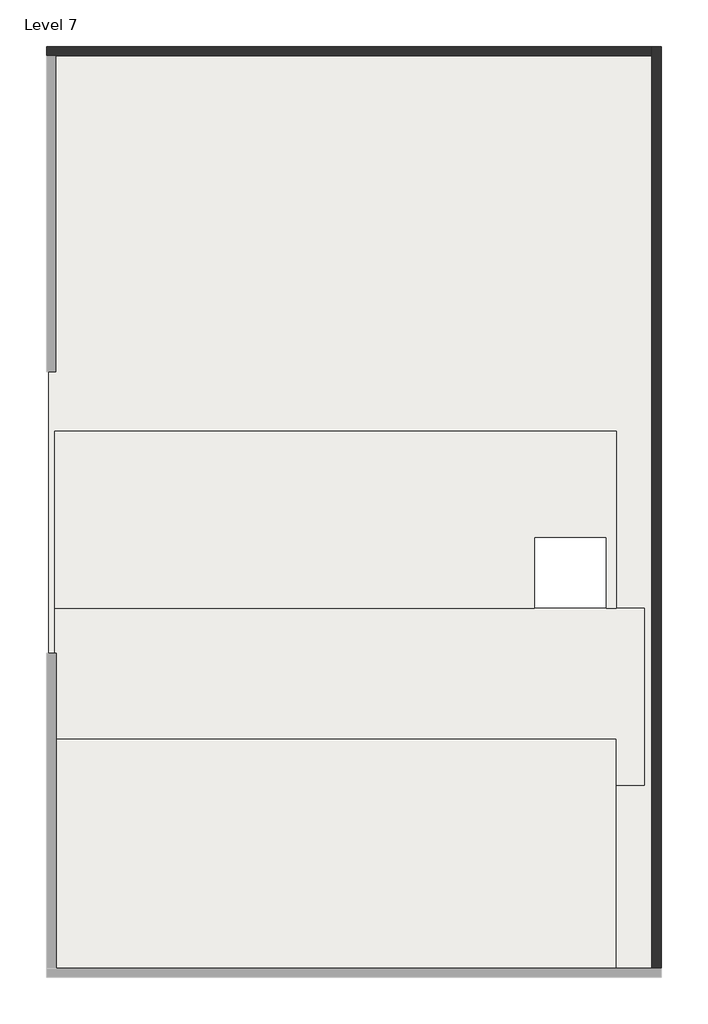
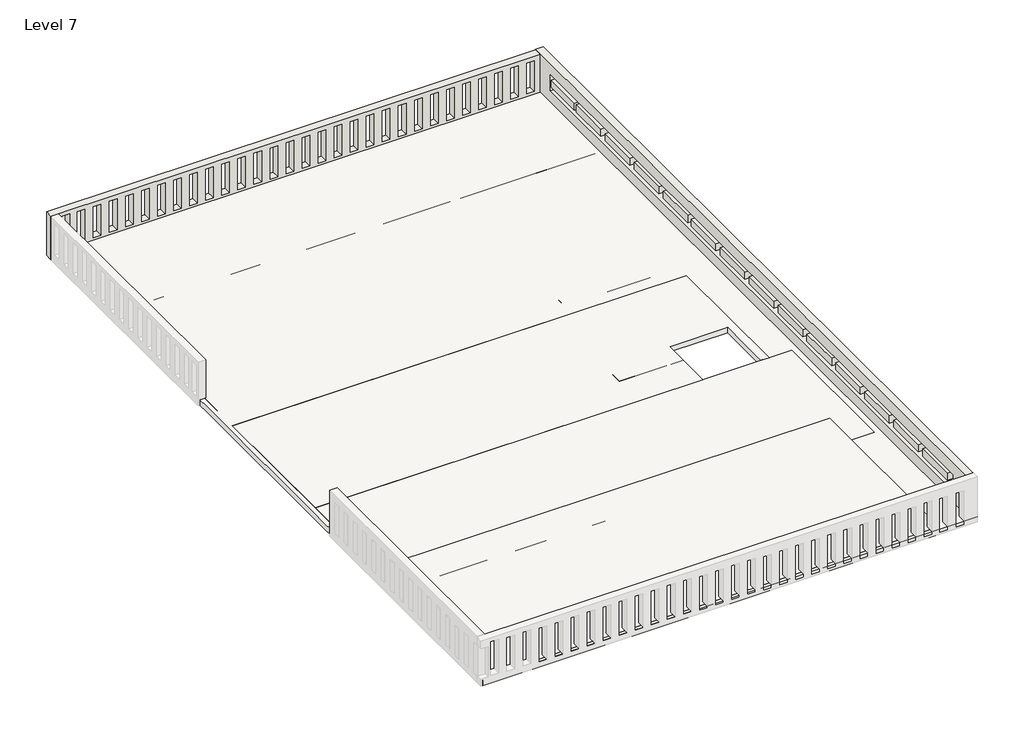
# One storey, part 2 of 2: 8 roofs, 2 walls.
"""IFC4 building model written with IfcOpenShell, lengths in millimetres."""

from ifc_helpers import new_model, si_unit, frame, origin, place, context, project, spatial, polyline, outline, extrude, faceted_brep, element, save

model = new_model("IFC4")

# Units and contexts
model_context = context("Model", 3, world=origin())
ifc_project = project(units=[si_unit("LENGTHUNIT", "METRE", prefix="MILLI")], contexts=[model_context])

# Site, building, storey
site = spatial("IfcSite", under=ifc_project)
building = spatial("IfcBuilding", under=site)
storey = spatial("IfcBuildingStorey", under=building, Name="Level 7", Elevation=18288.0)

# Roofs
placement = place(None, origin())
element("IfcRoof", 1, ObjectType="Generic - 12\"", at=placement, inside=storey, context=model_context, shape_type="SweptSolid", body=[
    extrude(outline(polyline([(-6354.2109037, 9427.2527313), (6498.1890963, 9427.2527313), (6498.1890963, 6506.6962251), (-6354.2109037, 6506.6962251), (-6354.2109037, 9427.2527313)])), frame((0.0, 0.0, 18288.0), z_axis=(0.0, 0.0, 1.0), x_axis=(1.0, 0.0, 0.0)), (0.0, 0.0, 1.0), 152.4),
])
element("IfcRoof", 2, ObjectType="Generic - 12\"", at=placement, inside=storey, context=model_context, shape_type="SweptSolid", body=[
    extrude(outline(polyline([(-6330.8013636, -2688.1037749), (6485.4890963, -2688.1037749), (6485.4890963, -6529.1251987), (-6330.8013636, -6529.1251987), (-6330.8013636, -2688.1037749)])), frame((0.0, 0.0, 18288.0), z_axis=(0.0, 0.0, 1.0), x_axis=(1.0, 0.0, 0.0)), (0.0, 0.0, 1.0), 152.4),
])
element("IfcRoof", 3, ObjectType="Generic - 12\"", at=placement, inside=storey, context=model_context, shape_type="SweptSolid", body=[
    extrude(outline(polyline([(-6354.2109037, -5532.9037749), (5863.1890963, -5532.9037749), (5863.1890963, -10612.9037749), (-6354.2109037, -10612.9037749), (-6354.2109037, -5532.9037749)])), frame((0.0, 0.0, 18288.0), z_axis=(0.0, 0.0, 1.0), x_axis=(1.0, 0.0, 0.0)), (0.0, 0.0, 1.0), 152.4),
])
element("IfcRoof", 4, ObjectType="Generic - 12\"", at=placement, inside=storey, context=model_context, shape_type="SweptSolid", body=[
    extrude(outline(polyline([(-6330.8013636, 6506.6962251), (5875.8890963, 6506.6962251), (5875.8890963, 1160.801054), (-6330.8013636, 1160.801054), (-6330.8013636, 6506.6962251)])), frame((0.0, 0.0, 18288.0), z_axis=(0.0, 0.0, 1.0), x_axis=(1.0, 0.0, 0.0)), (0.0, 0.0, 1.0), 152.4),
])
element("IfcRoof", 5, ObjectType="Generic - 12\"", at=placement, inside=storey, context=model_context, shape_type="SweptSolid", body=[
    extrude(outline(polyline([(-6330.8013636, 1160.801054), (5875.8890963, 1160.801054), (5875.8890963, -2688.1037749), (5659.9890963, -2688.1037749), (5659.9890963, -1138.7037749), (4097.8890963, -1138.7037749), (4097.8890963, -2688.1037749), (-6330.8013636, -2688.1037749), (-6330.8013636, 1160.801054)])), frame((0.0, 0.0, 18288.0), z_axis=(0.0, 0.0, 1.0), x_axis=(1.0, 0.0, 0.0)), (0.0, 0.0, 1.0), 152.4),
])
element("IfcRoof", 6, ObjectType="Generic - 12\"", at=placement, inside=storey, context=model_context, shape_type="SweptSolid", body=[
    extrude(outline(polyline([(2372.9046693, -1781.7441535), (2372.9046693, -1138.7037749), (4097.8890963, -1138.7037749), (4097.8890963, -1781.7441535), (2372.9046693, -1781.7441535)])), frame((0.0, 0.0, 18288.0), z_axis=(0.0, 0.0, 1.0), x_axis=(1.0, 0.0, 0.0)), (0.0, 0.0, 1.0), 152.4),
])
element("IfcRoof", 7, ObjectType="Generic - 12\"", at=placement, inside=storey, context=model_context, shape_type="SweptSolid", body=[
    extrude(outline(polyline([(5086.1735773, 1505.3140413), (2800.1735773, 1505.3140413), (2800.1735773, 1774.3862477), (5086.1735773, 1774.3862477), (5086.1735773, 1505.3140413)])), frame((0.0, 0.0, 18288.0), z_axis=(0.0, 0.0, 1.0), x_axis=(1.0, 0.0, 0.0)), (0.0, 0.0, 1.0), 152.4),
])
element("IfcRoof", 8, ObjectType="Generic - 12\"", at=placement, inside=storey, context=model_context, shape_type="SweptSolid", body=[
    extrude(outline(polyline([(6853.7890963, -10703.6694836), (-6455.8109037, -10703.6694836), (-6455.8109037, 9516.5962251), (6853.7890963, 9516.5962251), (6853.7890963, -10703.6694836)]), holes=[polyline([(5659.9890963, -1138.7037749), (4097.8890963, -1138.7037749), (4097.8890963, -2688.1037749), (5659.9890963, -2688.1037749), (5659.9890963, -1138.7037749)])]), frame((0.0, 0.0, 18288.0), z_axis=(0.0, 0.0, 1.0), x_axis=(1.0, 0.0, 0.0)), (0.0, 0.0, 1.0), 152.4),
])

# Walls
element("IfcWall", 9, ObjectType="Generic - 9\" w", at=placement, inside=storey, context=model_context, shape_type="Brep", body=[
    faceted_brep([(-6506.6109037, 9313.3962251, 18288.0), (-6303.4109037, 9313.3962251, 18288.0), (6650.5890963, 9313.3962251, 18288.0), (6650.5890963, 9313.3962251, 19521.0013439), (-6506.6109037, 9313.3962251, 19521.0013439), (-6506.6109037, 9313.3962251, 19520.2498043), (6294.9890963, 9313.3962251, 19391.3906419), (6498.1890963, 9313.3962251, 19391.3906419), (6498.1890963, 9313.3962251, 18512.6701562), (6294.9890963, 9313.3962251, 18512.6701562), (5863.1890963, 9313.3962251, 19391.3906419), (6066.3890963, 9313.3962251, 19391.3906419), (6066.3890963, 9313.3962251, 18512.6701562), (5863.1890963, 9313.3962251, 18512.6701562), (5431.3890963, 9313.3962251, 19391.3906419), (5634.5890963, 9313.3962251, 19391.3906419), (5634.5890963, 9313.3962251, 18512.6701562), (5431.3890963, 9313.3962251, 18512.6701562), (4999.5890963, 9313.3962251, 19391.3906419), (5202.7890963, 9313.3962251, 19391.3906419), (5202.7890963, 9313.3962251, 18512.6701562), (4999.5890963, 9313.3962251, 18512.6701562), (4567.7890963, 9313.3962251, 19391.3906419), (4770.9890963, 9313.3962251, 19391.3906419), (4770.9890963, 9313.3962251, 18512.6701562), (4567.7890963, 9313.3962251, 18512.6701562), (4135.9890963, 9313.3962251, 19391.3906419), (4339.1890963, 9313.3962251, 19391.3906419), (4339.1890963, 9313.3962251, 18512.6701562), (4135.9890963, 9313.3962251, 18512.6701562), (3704.1890963, 9313.3962251, 19391.3906419), (3907.3890963, 9313.3962251, 19391.3906419), (3907.3890963, 9313.3962251, 18512.6701562), (3704.1890963, 9313.3962251, 18512.6701562), (3272.3890963, 9313.3962251, 19391.3906419), (3475.5890963, 9313.3962251, 19391.3906419), (3475.5890963, 9313.3962251, 18512.6701562), (3272.3890963, 9313.3962251, 18512.6701562), (2840.5890963, 9313.3962251, 19391.3906419), (3043.7890963, 9313.3962251, 19391.3906419), (3043.7890963, 9313.3962251, 18512.6701562), (2840.5890963, 9313.3962251, 18512.6701562), (2408.7890963, 9313.3962251, 19391.3906419), (2611.9890963, 9313.3962251, 19391.3906419), (2611.9890963, 9313.3962251, 18512.6701562), (2408.7890963, 9313.3962251, 18512.6701562), (1976.9890963, 9313.3962251, 19391.3906419), (2180.1890963, 9313.3962251, 19391.3906419), (2180.1890963, 9313.3962251, 18512.6701562), (1976.9890963, 9313.3962251, 18512.6701562), (1545.1890963, 9313.3962251, 19391.3906419), (1748.3890963, 9313.3962251, 19391.3906419), (1748.3890963, 9313.3962251, 18512.6701562), (1545.1890963, 9313.3962251, 18512.6701562), (1113.3890963, 9313.3962251, 19391.3906419), (1316.5890963, 9313.3962251, 19391.3906419), (1316.5890963, 9313.3962251, 18512.6701562), (1113.3890963, 9313.3962251, 18512.6701562), (681.5890963, 9313.3962251, 19391.3906419), (884.7890963, 9313.3962251, 19391.3906419), (884.7890963, 9313.3962251, 18512.6701562), (681.5890963, 9313.3962251, 18512.6701562), (249.7890963, 9313.3962251, 19391.3906419), (452.9890963, 9313.3962251, 19391.3906419), (452.9890963, 9313.3962251, 18512.6701562), (249.7890963, 9313.3962251, 18512.6701562), (-182.0109037, 9313.3962251, 19391.3906419), (21.1890963, 9313.3962251, 19391.3906419), (21.1890963, 9313.3962251, 18512.6701562), (-182.0109037, 9313.3962251, 18512.6701562), (-613.8109037, 9313.3962251, 19391.3906419), (-410.6109037, 9313.3962251, 19391.3906419), (-410.6109037, 9313.3962251, 18512.6701562), (-613.8109037, 9313.3962251, 18512.6701562), (-1045.6109037, 9313.3962251, 19391.3906419), (-842.4109037, 9313.3962251, 19391.3906419), (-842.4109037, 9313.3962251, 18512.6701562), (-1045.6109037, 9313.3962251, 18512.6701562), (-1477.4109037, 9313.3962251, 19391.3906419), (-1274.2109037, 9313.3962251, 19391.3906419), (-1274.2109037, 9313.3962251, 18512.6701562), (-1477.4109037, 9313.3962251, 18512.6701562), (-1909.2109037, 9313.3962251, 19391.3906419), (-1706.0109037, 9313.3962251, 19391.3906419), (-1706.0109037, 9313.3962251, 18512.6701562), (-1909.2109037, 9313.3962251, 18512.6701562), (-2341.0109037, 9313.3962251, 19391.3906419), (-2137.8109037, 9313.3962251, 19391.3906419), (-2137.8109037, 9313.3962251, 18512.6701562), (-2341.0109037, 9313.3962251, 18512.6701562), (-2772.8109037, 9313.3962251, 19391.3906419), (-2569.6109037, 9313.3962251, 19391.3906419), (-2569.6109037, 9313.3962251, 18512.6701562), (-2772.8109037, 9313.3962251, 18512.6701562), (-3204.6109037, 9313.3962251, 19391.3906419), (-3001.4109037, 9313.3962251, 19391.3906419), (-3001.4109037, 9313.3962251, 18512.6701562), (-3204.6109037, 9313.3962251, 18512.6701562), (-3636.4109037, 9313.3962251, 19391.3906419), (-3433.2109037, 9313.3962251, 19391.3906419), (-3433.2109037, 9313.3962251, 18512.6701562), (-3636.4109037, 9313.3962251, 18512.6701562), (-4068.2109037, 9313.3962251, 19391.3906419), (-3865.0109037, 9313.3962251, 19391.3906419), (-3865.0109037, 9313.3962251, 18512.6701562), (-4068.2109037, 9313.3962251, 18512.6701562), (-4500.0109037, 9313.3962251, 19391.3906419), (-4296.8109037, 9313.3962251, 19391.3906419), (-4296.8109037, 9313.3962251, 18512.6701562), (-4500.0109037, 9313.3962251, 18512.6701562), (-4931.8109037, 9313.3962251, 19391.3906419), (-4728.6109037, 9313.3962251, 19391.3906419), (-4728.6109037, 9313.3962251, 18512.6701562), (-4931.8109037, 9313.3962251, 18512.6701562), (-5363.6109037, 9313.3962251, 19391.3906419), (-5160.4109037, 9313.3962251, 19391.3906419), (-5160.4109037, 9313.3962251, 18512.6701562), (-5363.6109037, 9313.3962251, 18512.6701562), (-5795.4109037, 9313.3962251, 19391.3906419), (-5592.2109037, 9313.3962251, 19391.3906419), (-5592.2109037, 9313.3962251, 18512.6701562), (-5795.4109037, 9313.3962251, 18512.6701562), (-6201.2539467, 9313.3962251, 19412.6599745), (-5998.0539467, 9313.3962251, 19412.6599745), (-5998.0539467, 9313.3962251, 18533.9394888), (-6201.2539467, 9313.3962251, 18533.9394888), (-6506.6109037, 9516.5962251, 18288.0), (-6506.6109037, 9516.5962251, 19521.0013439), (6650.5890963, 9516.5962251, 19521.0013439), (6650.5890963, 9516.5962251, 18288.0), (6294.9890963, 9516.5962251, 19391.3906419), (6294.9890963, 9516.5962251, 18512.6701562), (6498.1890963, 9516.5962251, 18512.6701562), (6498.1890963, 9516.5962251, 19391.3906419), (5863.1890963, 9516.5962251, 19391.3906419), (5863.1890963, 9516.5962251, 18512.6701562), (6066.3890963, 9516.5962251, 18512.6701562), (6066.3890963, 9516.5962251, 19391.3906419), (5431.3890963, 9516.5962251, 19391.3906419), (5431.3890963, 9516.5962251, 18512.6701562), (5634.5890963, 9516.5962251, 18512.6701562), (5634.5890963, 9516.5962251, 19391.3906419), (4999.5890963, 9516.5962251, 19391.3906419), (4999.5890963, 9516.5962251, 18512.6701562), (5202.7890963, 9516.5962251, 18512.6701562), (5202.7890963, 9516.5962251, 19391.3906419), (4567.7890963, 9516.5962251, 19391.3906419), (4567.7890963, 9516.5962251, 18512.6701562), (4770.9890963, 9516.5962251, 18512.6701562), (4770.9890963, 9516.5962251, 19391.3906419), (4135.9890963, 9516.5962251, 19391.3906419), (4135.9890963, 9516.5962251, 18512.6701562), (4339.1890963, 9516.5962251, 18512.6701562), (4339.1890963, 9516.5962251, 19391.3906419), (3704.1890963, 9516.5962251, 19391.3906419), (3704.1890963, 9516.5962251, 18512.6701562), (3907.3890963, 9516.5962251, 18512.6701562), (3907.3890963, 9516.5962251, 19391.3906419), (3272.3890963, 9516.5962251, 19391.3906419), (3272.3890963, 9516.5962251, 18512.6701562), (3475.5890963, 9516.5962251, 18512.6701562), (3475.5890963, 9516.5962251, 19391.3906419), (2840.5890963, 9516.5962251, 19391.3906419), (2840.5890963, 9516.5962251, 18512.6701562), (3043.7890963, 9516.5962251, 18512.6701562), (3043.7890963, 9516.5962251, 19391.3906419), (2408.7890963, 9516.5962251, 19391.3906419), (2408.7890963, 9516.5962251, 18512.6701562), (2611.9890963, 9516.5962251, 18512.6701562), (2611.9890963, 9516.5962251, 19391.3906419), (1976.9890963, 9516.5962251, 19391.3906419), (1976.9890963, 9516.5962251, 18512.6701562), (2180.1890963, 9516.5962251, 18512.6701562), (2180.1890963, 9516.5962251, 19391.3906419), (1545.1890963, 9516.5962251, 19391.3906419), (1545.1890963, 9516.5962251, 18512.6701562), (1748.3890963, 9516.5962251, 18512.6701562), (1748.3890963, 9516.5962251, 19391.3906419), (1113.3890963, 9516.5962251, 19391.3906419), (1113.3890963, 9516.5962251, 18512.6701562), (1316.5890963, 9516.5962251, 18512.6701562), (1316.5890963, 9516.5962251, 19391.3906419), (681.5890963, 9516.5962251, 19391.3906419), (681.5890963, 9516.5962251, 18512.6701562), (884.7890963, 9516.5962251, 18512.6701562), (884.7890963, 9516.5962251, 19391.3906419), (249.7890963, 9516.5962251, 19391.3906419), (249.7890963, 9516.5962251, 18512.6701562), (452.9890963, 9516.5962251, 18512.6701562), (452.9890963, 9516.5962251, 19391.3906419), (-182.0109037, 9516.5962251, 19391.3906419), (-182.0109037, 9516.5962251, 18512.6701562), (21.1890963, 9516.5962251, 18512.6701562), (21.1890963, 9516.5962251, 19391.3906419), (-613.8109037, 9516.5962251, 19391.3906419), (-613.8109037, 9516.5962251, 18512.6701562), (-410.6109037, 9516.5962251, 18512.6701562), (-410.6109037, 9516.5962251, 19391.3906419), (-1045.6109037, 9516.5962251, 19391.3906419), (-1045.6109037, 9516.5962251, 18512.6701562), (-842.4109037, 9516.5962251, 18512.6701562), (-842.4109037, 9516.5962251, 19391.3906419), (-1477.4109037, 9516.5962251, 19391.3906419), (-1477.4109037, 9516.5962251, 18512.6701562), (-1274.2109037, 9516.5962251, 18512.6701562), (-1274.2109037, 9516.5962251, 19391.3906419), (-1909.2109037, 9516.5962251, 19391.3906419), (-1909.2109037, 9516.5962251, 18512.6701562), (-1706.0109037, 9516.5962251, 18512.6701562), (-1706.0109037, 9516.5962251, 19391.3906419), (-2341.0109037, 9516.5962251, 19391.3906419), (-2341.0109037, 9516.5962251, 18512.6701562), (-2137.8109037, 9516.5962251, 18512.6701562), (-2137.8109037, 9516.5962251, 19391.3906419), (-2772.8109037, 9516.5962251, 19391.3906419), (-2772.8109037, 9516.5962251, 18512.6701562), (-2569.6109037, 9516.5962251, 18512.6701562), (-2569.6109037, 9516.5962251, 19391.3906419), (-3204.6109037, 9516.5962251, 19391.3906419), (-3204.6109037, 9516.5962251, 18512.6701562), (-3001.4109037, 9516.5962251, 18512.6701562), (-3001.4109037, 9516.5962251, 19391.3906419), (-3636.4109037, 9516.5962251, 19391.3906419), (-3636.4109037, 9516.5962251, 18512.6701562), (-3433.2109037, 9516.5962251, 18512.6701562), (-3433.2109037, 9516.5962251, 19391.3906419), (-4068.2109037, 9516.5962251, 19391.3906419), (-4068.2109037, 9516.5962251, 18512.6701562), (-3865.0109037, 9516.5962251, 18512.6701562), (-3865.0109037, 9516.5962251, 19391.3906419), (-4500.0109037, 9516.5962251, 19391.3906419), (-4500.0109037, 9516.5962251, 18512.6701562), (-4296.8109037, 9516.5962251, 18512.6701562), (-4296.8109037, 9516.5962251, 19391.3906419), (-4931.8109037, 9516.5962251, 19391.3906419), (-4931.8109037, 9516.5962251, 18512.6701562), (-4728.6109037, 9516.5962251, 18512.6701562), (-4728.6109037, 9516.5962251, 19391.3906419), (-5363.6109037, 9516.5962251, 19391.3906419), (-5363.6109037, 9516.5962251, 18512.6701562), (-5160.4109037, 9516.5962251, 18512.6701562), (-5160.4109037, 9516.5962251, 19391.3906419), (-5795.4109037, 9516.5962251, 19391.3906419), (-5795.4109037, 9516.5962251, 18512.6701562), (-5592.2109037, 9516.5962251, 18512.6701562), (-5592.2109037, 9516.5962251, 19391.3906419), (-6201.2539467, 9516.5962251, 19412.6599745), (-6201.2539467, 9516.5962251, 18533.9394888), (-5998.0539467, 9516.5962251, 18533.9394888), (-5998.0539467, 9516.5962251, 19412.6599745)], [[[0, 1, 2, 3, 4, 5], [6, 7, 8, 9], [10, 11, 12, 13], [14, 15, 16, 17], [18, 19, 20, 21], [22, 23, 24, 25], [26, 27, 28, 29], [30, 31, 32, 33], [34, 35, 36, 37], [38, 39, 40, 41], [42, 43, 44, 45], [46, 47, 48, 49], [50, 51, 52, 53], [54, 55, 56, 57], [58, 59, 60, 61], [62, 63, 64, 65], [66, 67, 68, 69], [70, 71, 72, 73], [74, 75, 76, 77], [78, 79, 80, 81], [82, 83, 84, 85], [86, 87, 88, 89], [90, 91, 92, 93], [94, 95, 96, 97], [98, 99, 100, 101], [102, 103, 104, 105], [106, 107, 108, 109], [110, 111, 112, 113], [114, 115, 116, 117], [118, 119, 120, 121], [122, 123, 124, 125]], [[126, 127, 128, 129], [130, 131, 132, 133], [134, 135, 136, 137], [138, 139, 140, 141], [142, 143, 144, 145], [146, 147, 148, 149], [150, 151, 152, 153], [154, 155, 156, 157], [158, 159, 160, 161], [162, 163, 164, 165], [166, 167, 168, 169], [170, 171, 172, 173], [174, 175, 176, 177], [178, 179, 180, 181], [182, 183, 184, 185], [186, 187, 188, 189], [190, 191, 192, 193], [194, 195, 196, 197], [198, 199, 200, 201], [202, 203, 204, 205], [206, 207, 208, 209], [210, 211, 212, 213], [214, 215, 216, 217], [218, 219, 220, 221], [222, 223, 224, 225], [226, 227, 228, 229], [230, 231, 232, 233], [234, 235, 236, 237], [238, 239, 240, 241], [242, 243, 244, 245], [246, 247, 248, 249]], [[3, 2, 129, 128]], [[2, 1, 0, 126, 129]], [[4, 3, 128, 127]], [[7, 6, 130, 133]], [[8, 7, 133, 132]], [[9, 8, 132, 131]], [[6, 9, 131, 130]], [[11, 10, 134, 137]], [[12, 11, 137, 136]], [[13, 12, 136, 135]], [[10, 13, 135, 134]], [[15, 14, 138, 141]], [[16, 15, 141, 140]], [[17, 16, 140, 139]], [[14, 17, 139, 138]], [[19, 18, 142, 145]], [[20, 19, 145, 144]], [[21, 20, 144, 143]], [[18, 21, 143, 142]], [[23, 22, 146, 149]], [[24, 23, 149, 148]], [[25, 24, 148, 147]], [[22, 25, 147, 146]], [[27, 26, 150, 153]], [[28, 27, 153, 152]], [[29, 28, 152, 151]], [[26, 29, 151, 150]], [[31, 30, 154, 157]], [[32, 31, 157, 156]], [[33, 32, 156, 155]], [[30, 33, 155, 154]], [[35, 34, 158, 161]], [[36, 35, 161, 160]], [[37, 36, 160, 159]], [[34, 37, 159, 158]], [[39, 38, 162, 165]], [[40, 39, 165, 164]], [[41, 40, 164, 163]], [[38, 41, 163, 162]], [[43, 42, 166, 169]], [[44, 43, 169, 168]], [[45, 44, 168, 167]], [[42, 45, 167, 166]], [[47, 46, 170, 173]], [[48, 47, 173, 172]], [[49, 48, 172, 171]], [[46, 49, 171, 170]], [[51, 50, 174, 177]], [[52, 51, 177, 176]], [[53, 52, 176, 175]], [[50, 53, 175, 174]], [[55, 54, 178, 181]], [[56, 55, 181, 180]], [[57, 56, 180, 179]], [[54, 57, 179, 178]], [[59, 58, 182, 185]], [[60, 59, 185, 184]], [[61, 60, 184, 183]], [[58, 61, 183, 182]], [[63, 62, 186, 189]], [[64, 63, 189, 188]], [[65, 64, 188, 187]], [[62, 65, 187, 186]], [[67, 66, 190, 193]], [[68, 67, 193, 192]], [[69, 68, 192, 191]], [[66, 69, 191, 190]], [[71, 70, 194, 197]], [[72, 71, 197, 196]], [[73, 72, 196, 195]], [[70, 73, 195, 194]], [[75, 74, 198, 201]], [[76, 75, 201, 200]], [[77, 76, 200, 199]], [[74, 77, 199, 198]], [[79, 78, 202, 205]], [[80, 79, 205, 204]], [[81, 80, 204, 203]], [[78, 81, 203, 202]], [[83, 82, 206, 209]], [[84, 83, 209, 208]], [[85, 84, 208, 207]], [[82, 85, 207, 206]], [[87, 86, 210, 213]], [[88, 87, 213, 212]], [[89, 88, 212, 211]], [[86, 89, 211, 210]], [[91, 90, 214, 217]], [[92, 91, 217, 216]], [[93, 92, 216, 215]], [[90, 93, 215, 214]], [[95, 94, 218, 221]], [[96, 95, 221, 220]], [[97, 96, 220, 219]], [[94, 97, 219, 218]], [[99, 98, 222, 225]], [[100, 99, 225, 224]], [[101, 100, 224, 223]], [[98, 101, 223, 222]], [[103, 102, 226, 229]], [[104, 103, 229, 228]], [[105, 104, 228, 227]], [[102, 105, 227, 226]], [[107, 106, 230, 233]], [[108, 107, 233, 232]], [[109, 108, 232, 231]], [[106, 109, 231, 230]], [[111, 110, 234, 237]], [[112, 111, 237, 236]], [[113, 112, 236, 235]], [[110, 113, 235, 234]], [[115, 114, 238, 241]], [[116, 115, 241, 240]], [[117, 116, 240, 239]], [[114, 117, 239, 238]], [[119, 118, 242, 245]], [[120, 119, 245, 244]], [[121, 120, 244, 243]], [[118, 121, 243, 242]], [[123, 122, 246, 249]], [[124, 123, 249, 248]], [[125, 124, 248, 247]], [[122, 125, 247, 246]], [[0, 5, 4, 127, 126]]]),
])
element("IfcWall", 10, ObjectType="Generic - 9\" w", at=placement, inside=storey, context=model_context, shape_type="Brep", body=[
    faceted_brep([(6650.5890963, 9516.5962251, 18288.0), (6650.5890963, 9313.3962251, 18288.0), (6650.5890963, -10500.4694836, 18288.0), (6650.5890963, -10500.4694836, 19542.6572919), (6650.5890963, 9516.5962251, 19542.6572919), (6650.5890963, 9516.5962251, 19521.0013439), (6650.5890963, 8837.1551186, 19224.3531832), (6650.5890963, -9908.0448814, 19224.3531832), (6650.5890963, -9908.0448814, 18767.1531832), (6650.5890963, 8837.1551186, 18767.1531832), (6853.7890963, 9516.5962251, 18288.0), (6853.7890963, 9516.5962251, 19542.6572919), (6853.7890963, -10500.4694836, 19542.6572919), (6853.7890963, -10500.4694836, 18288.0), (6853.7890963, 8837.1551186, 19224.3531832), (6853.7890963, 8837.1551186, 18767.1531832), (6853.7890963, -9908.0448814, 18767.1531832), (6853.7890963, -9908.0448814, 19224.3531832)], [[[0, 1, 2, 3, 4, 5], [6, 7, 8, 9]], [[10, 11, 12, 13], [14, 15, 16, 17]], [[0, 5, 4, 11, 10]], [[3, 2, 13, 12]], [[2, 1, 0, 10, 13]], [[4, 3, 12, 11]], [[7, 6, 14, 17]], [[8, 7, 17, 16]], [[9, 8, 16, 15]], [[6, 9, 15, 14]]]),
    faceted_brep([(6650.5890963, -8499.7753786, 19098.6118661), (6650.5890963, -8499.7753786, 18895.4118661), (6650.5890963, -9642.7753786, 18895.4118661), (6650.5890963, -9642.7753786, 19098.6118661), (6853.7890963, -8499.7753786, 19098.6118661), (6853.7890963, -9642.7753786, 19098.6118661), (6853.7890963, -9642.7753786, 18895.4118661), (6853.7890963, -8499.7753786, 18895.4118661)], [[[0, 1, 2, 3]], [[4, 5, 6, 7]], [[1, 0, 4, 7]], [[2, 1, 7, 6]], [[3, 2, 6, 5]], [[0, 3, 5, 4]]]),
    faceted_brep([(6650.5890963, -7153.5753786, 19098.6118661), (6650.5890963, -7153.5753786, 18895.4118661), (6650.5890963, -8296.5753786, 18895.4118661), (6650.5890963, -8296.5753786, 19098.6118661), (6853.7890963, -7153.5753786, 19098.6118661), (6853.7890963, -8296.5753786, 19098.6118661), (6853.7890963, -8296.5753786, 18895.4118661), (6853.7890963, -7153.5753786, 18895.4118661)], [[[0, 1, 2, 3]], [[4, 5, 6, 7]], [[1, 0, 4, 7]], [[2, 1, 7, 6]], [[3, 2, 6, 5]], [[0, 3, 5, 4]]]),
    faceted_brep([(6650.5890963, -5807.3753786, 19098.6118661), (6650.5890963, -5807.3753786, 18895.4118661), (6650.5890963, -6950.3753786, 18895.4118661), (6650.5890963, -6950.3753786, 19098.6118661), (6853.7890963, -5807.3753786, 19098.6118661), (6853.7890963, -6950.3753786, 19098.6118661), (6853.7890963, -6950.3753786, 18895.4118661), (6853.7890963, -5807.3753786, 18895.4118661)], [[[0, 1, 2, 3]], [[4, 5, 6, 7]], [[1, 0, 4, 7]], [[2, 1, 7, 6]], [[3, 2, 6, 5]], [[0, 3, 5, 4]]]),
    faceted_brep([(6650.5890963, -4461.1753786, 19098.6118661), (6650.5890963, -4461.1753786, 18895.4118661), (6650.5890963, -5604.1753786, 18895.4118661), (6650.5890963, -5604.1753786, 19098.6118661), (6853.7890963, -4461.1753786, 19098.6118661), (6853.7890963, -5604.1753786, 19098.6118661), (6853.7890963, -5604.1753786, 18895.4118661), (6853.7890963, -4461.1753786, 18895.4118661)], [[[0, 1, 2, 3]], [[4, 5, 6, 7]], [[1, 0, 4, 7]], [[2, 1, 7, 6]], [[3, 2, 6, 5]], [[0, 3, 5, 4]]]),
    faceted_brep([(6650.5890963, -3114.9753786, 19098.6118661), (6650.5890963, -3114.9753786, 18895.4118661), (6650.5890963, -4257.9753786, 18895.4118661), (6650.5890963, -4257.9753786, 19098.6118661), (6853.7890963, -3114.9753786, 19098.6118661), (6853.7890963, -4257.9753786, 19098.6118661), (6853.7890963, -4257.9753786, 18895.4118661), (6853.7890963, -3114.9753786, 18895.4118661)], [[[0, 1, 2, 3]], [[4, 5, 6, 7]], [[1, 0, 4, 7]], [[2, 1, 7, 6]], [[3, 2, 6, 5]], [[0, 3, 5, 4]]]),
    faceted_brep([(6650.5890963, -1768.7753786, 19098.6118661), (6650.5890963, -1768.7753786, 18895.4118661), (6650.5890963, -2911.7753786, 18895.4118661), (6650.5890963, -2911.7753786, 19098.6118661), (6853.7890963, -1768.7753786, 19098.6118661), (6853.7890963, -2911.7753786, 19098.6118661), (6853.7890963, -2911.7753786, 18895.4118661), (6853.7890963, -1768.7753786, 18895.4118661)], [[[0, 1, 2, 3]], [[4, 5, 6, 7]], [[1, 0, 4, 7]], [[2, 1, 7, 6]], [[3, 2, 6, 5]], [[0, 3, 5, 4]]]),
    faceted_brep([(6650.5890963, -422.5753786, 19098.6118661), (6650.5890963, -422.5753786, 18895.4118661), (6650.5890963, -1565.5753786, 18895.4118661), (6650.5890963, -1565.5753786, 19098.6118661), (6853.7890963, -422.5753786, 19098.6118661), (6853.7890963, -1565.5753786, 19098.6118661), (6853.7890963, -1565.5753786, 18895.4118661), (6853.7890963, -422.5753786, 18895.4118661)], [[[0, 1, 2, 3]], [[4, 5, 6, 7]], [[1, 0, 4, 7]], [[2, 1, 7, 6]], [[3, 2, 6, 5]], [[0, 3, 5, 4]]]),
    faceted_brep([(6650.5890963, 923.6246214, 19098.6118661), (6650.5890963, 923.6246214, 18895.4118661), (6650.5890963, -219.3753786, 18895.4118661), (6650.5890963, -219.3753786, 19098.6118661), (6853.7890963, 923.6246214, 19098.6118661), (6853.7890963, -219.3753786, 19098.6118661), (6853.7890963, -219.3753786, 18895.4118661), (6853.7890963, 923.6246214, 18895.4118661)], [[[0, 1, 2, 3]], [[4, 5, 6, 7]], [[1, 0, 4, 7]], [[2, 1, 7, 6]], [[3, 2, 6, 5]], [[0, 3, 5, 4]]]),
    faceted_brep([(6650.5890963, 2269.8246214, 19098.6118661), (6650.5890963, 2269.8246214, 18895.4118661), (6650.5890963, 1126.8246214, 18895.4118661), (6650.5890963, 1126.8246214, 19098.6118661), (6853.7890963, 2269.8246214, 19098.6118661), (6853.7890963, 1126.8246214, 19098.6118661), (6853.7890963, 1126.8246214, 18895.4118661), (6853.7890963, 2269.8246214, 18895.4118661)], [[[0, 1, 2, 3]], [[4, 5, 6, 7]], [[1, 0, 4, 7]], [[2, 1, 7, 6]], [[3, 2, 6, 5]], [[0, 3, 5, 4]]]),
    faceted_brep([(6650.5890963, 3590.6246214, 19098.6118661), (6650.5890963, 3590.6246214, 18895.4118661), (6650.5890963, 2447.6246214, 18895.4118661), (6650.5890963, 2447.6246214, 19098.6118661), (6853.7890963, 3590.6246214, 19098.6118661), (6853.7890963, 2447.6246214, 19098.6118661), (6853.7890963, 2447.6246214, 18895.4118661), (6853.7890963, 3590.6246214, 18895.4118661)], [[[0, 1, 2, 3]], [[4, 5, 6, 7]], [[1, 0, 4, 7]], [[2, 1, 7, 6]], [[3, 2, 6, 5]], [[0, 3, 5, 4]]]),
    faceted_brep([(6650.5890963, 4936.8246214, 19098.6118661), (6650.5890963, 4936.8246214, 18895.4118661), (6650.5890963, 3793.8246214, 18895.4118661), (6650.5890963, 3793.8246214, 19098.6118661), (6853.7890963, 4936.8246214, 19098.6118661), (6853.7890963, 3793.8246214, 19098.6118661), (6853.7890963, 3793.8246214, 18895.4118661), (6853.7890963, 4936.8246214, 18895.4118661)], [[[0, 1, 2, 3]], [[4, 5, 6, 7]], [[1, 0, 4, 7]], [[2, 1, 7, 6]], [[3, 2, 6, 5]], [[0, 3, 5, 4]]]),
    faceted_brep([(6650.5890963, 6283.0246214, 19098.6118661), (6650.5890963, 6283.0246214, 18895.4118661), (6650.5890963, 5140.0246214, 18895.4118661), (6650.5890963, 5140.0246214, 19098.6118661), (6853.7890963, 6283.0246214, 19098.6118661), (6853.7890963, 5140.0246214, 19098.6118661), (6853.7890963, 5140.0246214, 18895.4118661), (6853.7890963, 6283.0246214, 18895.4118661)], [[[0, 1, 2, 3]], [[4, 5, 6, 7]], [[1, 0, 4, 7]], [[2, 1, 7, 6]], [[3, 2, 6, 5]], [[0, 3, 5, 4]]]),
    faceted_brep([(6650.5890963, 7629.2246214, 19098.6118661), (6650.5890963, 7629.2246214, 18895.4118661), (6650.5890963, 6486.2246214, 18895.4118661), (6650.5890963, 6486.2246214, 19098.6118661), (6853.7890963, 7629.2246214, 19098.6118661), (6853.7890963, 6486.2246214, 19098.6118661), (6853.7890963, 6486.2246214, 18895.4118661), (6853.7890963, 7629.2246214, 18895.4118661)], [[[0, 1, 2, 3]], [[4, 5, 6, 7]], [[1, 0, 4, 7]], [[2, 1, 7, 6]], [[3, 2, 6, 5]], [[0, 3, 5, 4]]]),
    faceted_brep([(6650.5890963, 8787.614598, 19098.6118661), (6650.5890963, 8787.614598, 18895.4118661), (6650.5890963, 7716.6518079, 18895.4118661), (6650.5890963, 7716.6518079, 19098.6118661), (6853.7890963, 8787.614598, 19098.6118661), (6853.7890963, 7716.6518079, 19098.6118661), (6853.7890963, 7716.6518079, 18895.4118661), (6853.7890963, 8787.614598, 18895.4118661)], [[[0, 1, 2, 3]], [[4, 5, 6, 7]], [[1, 0, 4, 7]], [[2, 1, 7, 6]], [[3, 2, 6, 5]], [[0, 3, 5, 4]]]),
])

save(model, "model.ifc")

# Revit data of these elements
# Type "Generic - 12\""
#   Assembly Code = "B1020"
#   Layers, outside or top first: 0' - 6" no material (function 1)
# Type "Generic - 9\" w"
#   Assembly Code = "B2010"
#   Layers, outside or top first: 0' - 8" no material (function 1)
# Element 1 (IfcRoof, "Generic - 12\"")
#   built-in parameter 1001705 = 60.5 (stored number, unit not read)
#   built-in parameter 1001710 = 33615
#   Phase Created = New Construction
#   Materials on its faces: "Default Roof", "Metal Furring"
# Elements 2, 3, 4, 6, 7 (IfcRoof, "Generic - 12\"")
#   built-in parameter 1001705 = 60.5 (stored number, unit not read)
#   built-in parameter 1001710 = 33615
#   Phase Created = New Construction
#   Materials on its faces: "Default Roof"
# Element 5 (IfcRoof, "Generic - 12\"")
#   built-in parameter 1001705 = 60.5 (stored number, unit not read)
#   built-in parameter 1001710 = 33615
#   Phase Created = New Construction
#   Materials on its faces: "Default Roof", "Default Mass Zone"
# Element 8 (IfcRoof, "Generic - 12\"")
#   built-in parameter 1001705 = 60.5 (stored number, unit not read)
#   built-in parameter 1001710 = 33615
#   Phase Created = New Construction
#   Materials on its faces: "Default Roof", "Aluminum"
# Element 9 (IfcWall, "Generic - 9\" w")
#   Top Offset = 0' - 0"
#   Base Offset = 0' - 0"
#   Unconnected Height = 4' - 0.54336"
#   wall height = 4' - 0.54336"
#   Phase Created = New Construction
#   Base Constraint = Level 7
#   Materials on its faces: "Default Wall", "Metal Furring", "Area Loads"
# Element 10 (IfcWall, "Generic - 9\" w")
#   Top Offset = 0' - 0"
#   Base Offset = 0' - 0"
#   Unconnected Height = 4' - 1.39596"
#   wall height = 4' - 1.39596"
#   Phase Created = New Construction
#   Base Constraint = Level 7
#   Materials on its faces: "Default Wall", "Metal Furring"
# Materials
#   "Default Roof": colour RGB 88 101 114, transparency 0, Cost = 0
#   "Metal Furring": class "Metal", colour RGB 199 199 199, transparency 0, Description = "Light gauge steel furring", Cost = 0
#   "Default Mass Zone": class "Generic", colour RGB 74 74 255, transparency 0.5, Cost = 0
#   "Aluminum": class "Metal", colour RGB 247 247 247, transparency 0, Description = "Aluminum 6061", Cost = 0
#   "Default Wall": colour RGB 128 128 128, transparency 0, Cost = 0
#   "Area Loads": colour RGB 191 178 255, transparency 0.5
